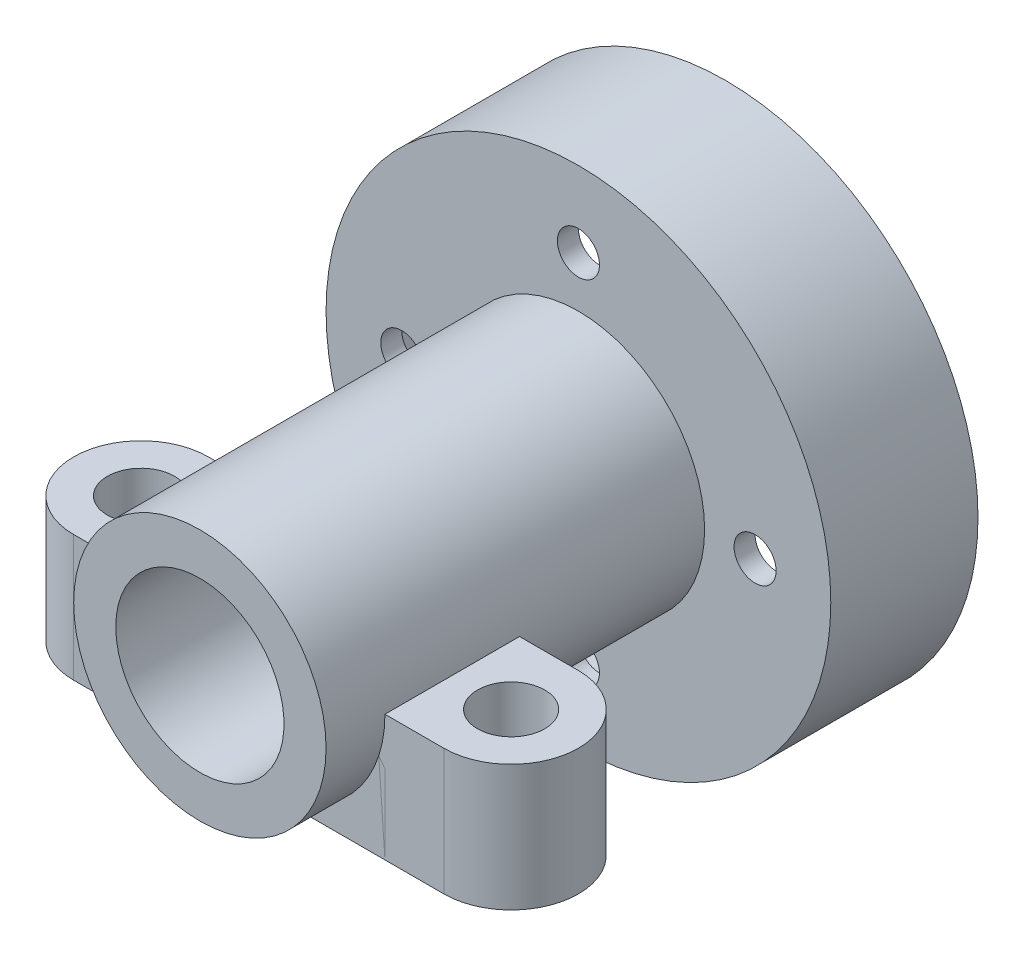
ISO-10303-21;
HEADER;
FILE_DESCRIPTION(('STEP AP214'),'2;1');
FILE_NAME('part.step','',(''),(''),'','','');
FILE_SCHEMA(('AUTOMOTIVE_DESIGN { 1 0 10303 214 1 1 1 1 }'));
ENDSEC;
DATA;
#1=APPLICATION_CONTEXT('core data for automotive mechanical design processes');
#2=APPLICATION_PROTOCOL_DEFINITION('international standard','automotive_design',2000,#1);
#3=PRODUCT_CONTEXT('',#1,'mechanical');
#4=PRODUCT('Part','Part','',(#3));
#5=PRODUCT_RELATED_PRODUCT_CATEGORY('part','',(#4));
#6=PRODUCT_DEFINITION_FORMATION('','',#4);
#7=PRODUCT_DEFINITION_CONTEXT('part definition',#1,'design');
#8=PRODUCT_DEFINITION('design','',#6,#7);
#9=PRODUCT_DEFINITION_SHAPE('','',#8);
#10=(LENGTH_UNIT() NAMED_UNIT(*) SI_UNIT(.MILLI.,.METRE.));
#11=(NAMED_UNIT(*) PLANE_ANGLE_UNIT() SI_UNIT($,.RADIAN.));
#12=(NAMED_UNIT(*) SI_UNIT($,.STERADIAN.) SOLID_ANGLE_UNIT());
#13=UNCERTAINTY_MEASURE_WITH_UNIT(LENGTH_MEASURE(1.E-05),#10,'distance_accuracy_value','');
#14=(GEOMETRIC_REPRESENTATION_CONTEXT(3) GLOBAL_UNCERTAINTY_ASSIGNED_CONTEXT((#13)) GLOBAL_UNIT_ASSIGNED_CONTEXT((#10,
#11,#12)) REPRESENTATION_CONTEXT('',''));
#15=CARTESIAN_POINT('',(0.,0.,0.));
#16=DIRECTION('',(0.,0.,1.));
#17=DIRECTION('',(1.,0.,0.));
#18=AXIS2_PLACEMENT_3D('',#15,#16,#17);
#19=CARTESIAN_POINT('',(0.,0.,81.));
#20=DIRECTION('',(0.,0.,1.));
#21=DIRECTION('',(1.,0.,0.));
#22=AXIS2_PLACEMENT_3D('',#19,#20,#21);
#23=CYLINDRICAL_SURFACE('',#22,30.);
#24=CARTESIAN_POINT('',(0.,0.,111.));
#25=DIRECTION('',(0.,0.,1.));
#26=DIRECTION('',(1.,0.,0.));
#27=AXIS2_PLACEMENT_3D('',#24,#25,#26);
#28=CIRCLE('',#27,30.);
#29=CARTESIAN_POINT('',(0.,-30.,111.));
#30=VERTEX_POINT('',#29);
#31=CARTESIAN_POINT('',(30.,0.,111.));
#32=VERTEX_POINT('',#31);
#33=EDGE_CURVE('E13',#30,#32,#28,.T.);
#34=ORIENTED_EDGE('',*,*,#33,.T.);
#35=DIRECTION('',(0.,0.,1.));
#36=VECTOR('',#35,1.);
#37=CARTESIAN_POINT('',(30.,0.,81.));
#38=LINE('',#37,#36);
#39=CARTESIAN_POINT('',(30.,0.,81.));
#40=VERTEX_POINT('',#39);
#41=EDGE_CURVE('E136',#40,#32,#38,.T.);
#42=ORIENTED_EDGE('',*,*,#41,.F.);
#43=CARTESIAN_POINT('',(0.,0.,81.));
#44=DIRECTION('',(0.,0.,1.));
#45=DIRECTION('',(1.,0.,0.));
#46=AXIS2_PLACEMENT_3D('',#43,#44,#45);
#47=CIRCLE('',#46,30.);
#48=CARTESIAN_POINT('',(0.,-30.,81.));
#49=VERTEX_POINT('',#48);
#50=EDGE_CURVE('E140',#49,#40,#47,.T.);
#51=ORIENTED_EDGE('',*,*,#50,.F.);
#52=DIRECTION('',(0.,0.,1.));
#53=VECTOR('',#52,1.);
#54=CARTESIAN_POINT('',(0.,-30.,81.));
#55=LINE('',#54,#53);
#56=EDGE_CURVE('E95',#49,#30,#55,.T.);
#57=ORIENTED_EDGE('',*,*,#56,.T.);
#58=EDGE_LOOP('',(#34,#42,#51,#57));
#59=FACE_BOUND('',#58,.T.);
#60=ADVANCED_FACE('F89',(#59),#23,.F.);
#61=CARTESIAN_POINT('',(30.,0.,81.));
#62=DIRECTION('',(-1.,0.,0.));
#63=DIRECTION('',(0.,0.,1.));
#64=AXIS2_PLACEMENT_3D('',#61,#62,#63);
#65=PLANE('',#64);
#66=DIRECTION('',(0.,-1.,0.));
#67=VECTOR('',#66,1.);
#68=CARTESIAN_POINT('',(30.,0.,111.));
#69=LINE('',#68,#67);
#70=CARTESIAN_POINT('',(30.,-30.,111.));
#71=VERTEX_POINT('',#70);
#72=EDGE_CURVE('E132',#32,#71,#69,.T.);
#73=ORIENTED_EDGE('',*,*,#72,.T.);
#74=DIRECTION('',(0.,0.,1.));
#75=VECTOR('',#74,1.);
#76=CARTESIAN_POINT('',(30.,-30.,81.));
#77=LINE('',#76,#75);
#78=CARTESIAN_POINT('',(30.,-30.,81.));
#79=VERTEX_POINT('',#78);
#80=EDGE_CURVE('E107',#79,#71,#77,.T.);
#81=ORIENTED_EDGE('',*,*,#80,.F.);
#82=DIRECTION('',(0.,-1.,0.));
#83=VECTOR('',#82,1.);
#84=CARTESIAN_POINT('',(30.,0.,81.));
#85=LINE('',#84,#83);
#86=EDGE_CURVE('E119',#40,#79,#85,.T.);
#87=ORIENTED_EDGE('',*,*,#86,.F.);
#88=ORIENTED_EDGE('',*,*,#41,.T.);
#89=EDGE_LOOP('',(#73,#81,#87,#88));
#90=FACE_BOUND('',#89,.T.);
#91=ADVANCED_FACE('F147',(#90),#65,.F.);
#92=CARTESIAN_POINT('',(0.,-30.,81.));
#93=DIRECTION('',(0.,-1.,0.));
#94=DIRECTION('',(0.,0.,-1.));
#95=AXIS2_PLACEMENT_3D('',#92,#93,#94);
#96=PLANE('',#95);
#97=DIRECTION('',(1.,0.,0.));
#98=VECTOR('',#97,1.);
#99=CARTESIAN_POINT('',(0.,-30.,111.));
#100=LINE('',#99,#98);
#101=EDGE_CURVE('E99',#30,#71,#100,.T.);
#102=ORIENTED_EDGE('',*,*,#101,.F.);
#103=ORIENTED_EDGE('',*,*,#56,.F.);
#104=DIRECTION('',(1.,0.,0.));
#105=VECTOR('',#104,1.);
#106=CARTESIAN_POINT('',(0.,-30.,81.));
#107=LINE('',#106,#105);
#108=EDGE_CURVE('E123',#49,#79,#107,.T.);
#109=ORIENTED_EDGE('',*,*,#108,.T.);
#110=ORIENTED_EDGE('',*,*,#80,.T.);
#111=EDGE_LOOP('',(#102,#103,#109,#110));
#112=FACE_BOUND('',#111,.T.);
#113=ADVANCED_FACE('F133',(#112),#96,.T.);
#114=CARTESIAN_POINT('',(0.,0.,81.));
#115=DIRECTION('',(0.,0.,1.));
#116=DIRECTION('',(1.,0.,0.));
#117=AXIS2_PLACEMENT_3D('',#114,#115,#116);
#118=PLANE('',#117);
#119=ORIENTED_EDGE('',*,*,#50,.T.);
#120=ORIENTED_EDGE('',*,*,#86,.T.);
#121=ORIENTED_EDGE('',*,*,#108,.F.);
#122=EDGE_LOOP('',(#119,#120,#121));
#123=FACE_BOUND('',#122,.T.);
#124=ADVANCED_FACE('F94',(#123),#118,.F.);
#125=CARTESIAN_POINT('',(0.,0.,111.));
#126=DIRECTION('',(0.,0.,1.));
#127=DIRECTION('',(1.,0.,0.));
#128=AXIS2_PLACEMENT_3D('',#125,#126,#127);
#129=PLANE('',#128);
#130=ORIENTED_EDGE('',*,*,#33,.F.);
#131=ORIENTED_EDGE('',*,*,#101,.T.);
#132=ORIENTED_EDGE('',*,*,#72,.F.);
#133=EDGE_LOOP('',(#130,#131,#132));
#134=FACE_BOUND('',#133,.T.);
#135=ADVANCED_FACE('F138',(#134),#129,.T.);
#136=CLOSED_SHELL('',(#60,#91,#113,#124,#135));
#137=MANIFOLD_SOLID_BREP('B2',#136);
#138=CARTESIAN_POINT('',(0.,0.,81.));
#139=DIRECTION('',(0.,0.,1.));
#140=DIRECTION('',(1.,0.,0.));
#141=AXIS2_PLACEMENT_3D('',#138,#139,#140);
#142=CYLINDRICAL_SURFACE('',#141,30.);
#143=CARTESIAN_POINT('',(0.,0.,111.));
#144=DIRECTION('',(0.,0.,1.));
#145=DIRECTION('',(1.,0.,0.));
#146=AXIS2_PLACEMENT_3D('',#143,#144,#145);
#147=CIRCLE('',#146,30.);
#148=CARTESIAN_POINT('',(-30.,0.,111.));
#149=VERTEX_POINT('',#148);
#150=CARTESIAN_POINT('',(0.,-30.,111.));
#151=VERTEX_POINT('',#150);
#152=EDGE_CURVE('E242',#149,#151,#147,.T.);
#153=ORIENTED_EDGE('',*,*,#152,.T.);
#154=DIRECTION('',(0.,0.,1.));
#155=VECTOR('',#154,1.);
#156=CARTESIAN_POINT('',(0.,-30.,81.));
#157=LINE('',#156,#155);
#158=CARTESIAN_POINT('',(0.,-30.,81.));
#159=VERTEX_POINT('',#158);
#160=EDGE_CURVE('E86',#159,#151,#157,.T.);
#161=ORIENTED_EDGE('',*,*,#160,.F.);
#162=CARTESIAN_POINT('',(0.,0.,81.));
#163=DIRECTION('',(0.,0.,1.));
#164=DIRECTION('',(1.,0.,0.));
#165=AXIS2_PLACEMENT_3D('',#162,#163,#164);
#166=CIRCLE('',#165,30.);
#167=CARTESIAN_POINT('',(-30.,0.,81.));
#168=VERTEX_POINT('',#167);
#169=EDGE_CURVE('E250',#168,#159,#166,.T.);
#170=ORIENTED_EDGE('',*,*,#169,.F.);
#171=DIRECTION('',(0.,0.,1.));
#172=VECTOR('',#171,1.);
#173=CARTESIAN_POINT('',(-30.,0.,81.));
#174=LINE('',#173,#172);
#175=EDGE_CURVE('E202',#168,#149,#174,.T.);
#176=ORIENTED_EDGE('',*,*,#175,.T.);
#177=EDGE_LOOP('',(#153,#161,#170,#176));
#178=FACE_BOUND('',#177,.T.);
#179=ADVANCED_FACE('F199',(#178),#142,.F.);
#180=CARTESIAN_POINT('',(0.,-30.,81.));
#181=DIRECTION('',(0.,-1.,0.));
#182=DIRECTION('',(0.,0.,-1.));
#183=AXIS2_PLACEMENT_3D('',#180,#181,#182);
#184=PLANE('',#183);
#185=DIRECTION('',(1.,0.,0.));
#186=VECTOR('',#185,1.);
#187=CARTESIAN_POINT('',(0.,-30.,111.));
#188=LINE('',#187,#186);
#189=CARTESIAN_POINT('',(-30.,-30.,111.));
#190=VERTEX_POINT('',#189);
#191=EDGE_CURVE('E243',#190,#151,#188,.T.);
#192=ORIENTED_EDGE('',*,*,#191,.F.);
#193=DIRECTION('',(0.,0.,1.));
#194=VECTOR('',#193,1.);
#195=CARTESIAN_POINT('',(-30.,-30.,81.));
#196=LINE('',#195,#194);
#197=CARTESIAN_POINT('',(-30.,-30.,81.));
#198=VERTEX_POINT('',#197);
#199=EDGE_CURVE('E209',#198,#190,#196,.T.);
#200=ORIENTED_EDGE('',*,*,#199,.F.);
#201=DIRECTION('',(1.,0.,0.));
#202=VECTOR('',#201,1.);
#203=CARTESIAN_POINT('',(0.,-30.,81.));
#204=LINE('',#203,#202);
#205=EDGE_CURVE('E254',#198,#159,#204,.T.);
#206=ORIENTED_EDGE('',*,*,#205,.T.);
#207=ORIENTED_EDGE('',*,*,#160,.T.);
#208=EDGE_LOOP('',(#192,#200,#206,#207));
#209=FACE_BOUND('',#208,.T.);
#210=ADVANCED_FACE('F246',(#209),#184,.T.);
#211=CARTESIAN_POINT('',(-30.,0.,81.));
#212=DIRECTION('',(-1.,0.,0.));
#213=DIRECTION('',(0.,0.,1.));
#214=AXIS2_PLACEMENT_3D('',#211,#212,#213);
#215=PLANE('',#214);
#216=DIRECTION('',(0.,-1.,0.));
#217=VECTOR('',#216,1.);
#218=CARTESIAN_POINT('',(-30.,0.,111.));
#219=LINE('',#218,#217);
#220=EDGE_CURVE('E234',#149,#190,#219,.T.);
#221=ORIENTED_EDGE('',*,*,#220,.F.);
#222=ORIENTED_EDGE('',*,*,#175,.F.);
#223=DIRECTION('',(0.,-1.,0.));
#224=VECTOR('',#223,1.);
#225=CARTESIAN_POINT('',(-30.,0.,81.));
#226=LINE('',#225,#224);
#227=EDGE_CURVE('E236',#168,#198,#226,.T.);
#228=ORIENTED_EDGE('',*,*,#227,.T.);
#229=ORIENTED_EDGE('',*,*,#199,.T.);
#230=EDGE_LOOP('',(#221,#222,#228,#229));
#231=FACE_BOUND('',#230,.T.);
#232=ADVANCED_FACE('F231',(#231),#215,.T.);
#233=CARTESIAN_POINT('',(0.,0.,81.));
#234=DIRECTION('',(0.,0.,1.));
#235=DIRECTION('',(1.,0.,0.));
#236=AXIS2_PLACEMENT_3D('',#233,#234,#235);
#237=PLANE('',#236);
#238=ORIENTED_EDGE('',*,*,#169,.T.);
#239=ORIENTED_EDGE('',*,*,#205,.F.);
#240=ORIENTED_EDGE('',*,*,#227,.F.);
#241=EDGE_LOOP('',(#238,#239,#240));
#242=FACE_BOUND('',#241,.T.);
#243=ADVANCED_FACE('F257',(#242),#237,.F.);
#244=CARTESIAN_POINT('',(0.,0.,111.));
#245=DIRECTION('',(0.,0.,1.));
#246=DIRECTION('',(1.,0.,0.));
#247=AXIS2_PLACEMENT_3D('',#244,#245,#246);
#248=PLANE('',#247);
#249=ORIENTED_EDGE('',*,*,#152,.F.);
#250=ORIENTED_EDGE('',*,*,#220,.T.);
#251=ORIENTED_EDGE('',*,*,#191,.T.);
#252=EDGE_LOOP('',(#249,#250,#251));
#253=FACE_BOUND('',#252,.T.);
#254=ADVANCED_FACE('F245',(#253),#248,.T.);
#255=CLOSED_SHELL('',(#179,#210,#232,#243,#254));
#256=MANIFOLD_SOLID_BREP('B7',#255);
#257=CARTESIAN_POINT('',(0.,0.,65.));
#258=DIRECTION('',(0.,0.,-1.));
#259=DIRECTION('',(-1.,0.,0.));
#260=AXIS2_PLACEMENT_3D('',#257,#258,#259);
#261=CYLINDRICAL_SURFACE('',#260,30.);
#262=CARTESIAN_POINT('',(0.,0.,35.));
#263=DIRECTION('',(0.,0.,1.));
#264=DIRECTION('',(1.,0.,0.));
#265=AXIS2_PLACEMENT_3D('',#262,#263,#264);
#266=CIRCLE('',#265,30.);
#267=CARTESIAN_POINT('',(30.,0.,35.));
#268=VERTEX_POINT('',#267);
#269=EDGE_CURVE('E362',#268,#268,#266,.T.);
#270=ORIENTED_EDGE('',*,*,#269,.T.);
#271=EDGE_LOOP('',(#270));
#272=FACE_BOUND('',#271,.T.);
#273=CARTESIAN_POINT('',(0.,0.,125.));
#274=DIRECTION('',(0.,0.,1.));
#275=DIRECTION('',(1.,0.,0.));
#276=AXIS2_PLACEMENT_3D('',#273,#274,#275);
#277=CIRCLE('',#276,30.);
#278=CARTESIAN_POINT('',(30.,0.,125.));
#279=VERTEX_POINT('',#278);
#280=EDGE_CURVE('E401',#279,#279,#277,.T.);
#281=ORIENTED_EDGE('',*,*,#280,.F.);
#282=EDGE_LOOP('',(#281));
#283=FACE_BOUND('',#282,.T.);
#284=CARTESIAN_POINT('',(0.,0.,79.));
#285=DIRECTION('',(0.,0.,1.));
#286=DIRECTION('',(1.,0.,0.));
#287=AXIS2_PLACEMENT_3D('',#284,#285,#286);
#288=CIRCLE('',#287,30.);
#289=CARTESIAN_POINT('',(-30.,0.,79.));
#290=VERTEX_POINT('',#289);
#291=CARTESIAN_POINT('',(0.,-30.,79.));
#292=VERTEX_POINT('',#291);
#293=EDGE_CURVE('E432',#290,#292,#288,.T.);
#294=ORIENTED_EDGE('',*,*,#293,.F.);
#295=DIRECTION('',(0.,0.,1.));
#296=VECTOR('',#295,1.);
#297=CARTESIAN_POINT('',(-30.,0.,79.));
#298=LINE('',#297,#296);
#299=CARTESIAN_POINT('',(-30.,0.,111.));
#300=VERTEX_POINT('',#299);
#301=EDGE_CURVE('E430',#290,#300,#298,.T.);
#302=ORIENTED_EDGE('',*,*,#301,.T.);
#303=CARTESIAN_POINT('',(0.,0.,111.));
#304=DIRECTION('',(0.,0.,1.));
#305=DIRECTION('',(1.,0.,0.));
#306=AXIS2_PLACEMENT_3D('',#303,#304,#305);
#307=CIRCLE('',#306,30.);
#308=CARTESIAN_POINT('',(0.,-30.,111.));
#309=VERTEX_POINT('',#308);
#310=EDGE_CURVE('E434',#300,#309,#307,.T.);
#311=ORIENTED_EDGE('',*,*,#310,.T.);
#312=CARTESIAN_POINT('',(0.,0.,111.));
#313=DIRECTION('',(0.,0.,1.));
#314=DIRECTION('',(1.,0.,0.));
#315=AXIS2_PLACEMENT_3D('',#312,#313,#314);
#316=CIRCLE('',#315,30.);
#317=CARTESIAN_POINT('',(30.,0.,111.));
#318=VERTEX_POINT('',#317);
#319=EDGE_CURVE('E326',#309,#318,#316,.T.);
#320=ORIENTED_EDGE('',*,*,#319,.T.);
#321=DIRECTION('',(0.,0.,1.));
#322=VECTOR('',#321,1.);
#323=CARTESIAN_POINT('',(30.,0.,79.));
#324=LINE('',#323,#322);
#325=CARTESIAN_POINT('',(30.,0.,79.));
#326=VERTEX_POINT('',#325);
#327=EDGE_CURVE('E350',#326,#318,#324,.T.);
#328=ORIENTED_EDGE('',*,*,#327,.F.);
#329=CARTESIAN_POINT('',(0.,0.,79.));
#330=DIRECTION('',(0.,0.,1.));
#331=DIRECTION('',(1.,0.,0.));
#332=AXIS2_PLACEMENT_3D('',#329,#330,#331);
#333=CIRCLE('',#332,30.);
#334=EDGE_CURVE('E363',#292,#326,#333,.T.);
#335=ORIENTED_EDGE('',*,*,#334,.F.);
#336=EDGE_LOOP('',(#294,#302,#311,#320,#328,#335));
#337=FACE_BOUND('',#336,.T.);
#338=ADVANCED_FACE('F296',(#272,#283,#337),#261,.T.);
#339=CARTESIAN_POINT('',(44.,-30.,95.));
#340=DIRECTION('',(0.,1.,0.));
#341=DIRECTION('',(0.,0.,1.));
#342=AXIS2_PLACEMENT_3D('',#339,#340,#341);
#343=CYLINDRICAL_SURFACE('',#342,16.);
#344=CARTESIAN_POINT('',(44.,0.,95.));
#345=DIRECTION('',(0.,1.,0.));
#346=DIRECTION('',(0.,0.,1.));
#347=AXIS2_PLACEMENT_3D('',#344,#345,#346);
#348=CIRCLE('',#347,16.);
#349=CARTESIAN_POINT('',(44.,0.,111.));
#350=VERTEX_POINT('',#349);
#351=CARTESIAN_POINT('',(44.,0.,79.));
#352=VERTEX_POINT('',#351);
#353=EDGE_CURVE('E339',#350,#352,#348,.T.);
#354=ORIENTED_EDGE('',*,*,#353,.F.);
#355=DIRECTION('',(0.,1.,0.));
#356=VECTOR('',#355,1.);
#357=CARTESIAN_POINT('',(44.,-30.,111.));
#358=LINE('',#357,#356);
#359=CARTESIAN_POINT('',(44.,-30.,111.));
#360=VERTEX_POINT('',#359);
#361=EDGE_CURVE('E196',#360,#350,#358,.T.);
#362=ORIENTED_EDGE('',*,*,#361,.F.);
#363=CARTESIAN_POINT('',(44.,-30.,95.));
#364=DIRECTION('',(0.,1.,0.));
#365=DIRECTION('',(0.,0.,1.));
#366=AXIS2_PLACEMENT_3D('',#363,#364,#365);
#367=CIRCLE('',#366,16.);
#368=CARTESIAN_POINT('',(44.,-30.,79.));
#369=VERTEX_POINT('',#368);
#370=EDGE_CURVE('E346',#360,#369,#367,.T.);
#371=ORIENTED_EDGE('',*,*,#370,.T.);
#372=DIRECTION('',(0.,1.,0.));
#373=VECTOR('',#372,1.);
#374=CARTESIAN_POINT('',(44.,-30.,79.));
#375=LINE('',#374,#373);
#376=EDGE_CURVE('E305',#369,#352,#375,.T.);
#377=ORIENTED_EDGE('',*,*,#376,.T.);
#378=EDGE_LOOP('',(#354,#362,#371,#377));
#379=FACE_BOUND('',#378,.T.);
#380=ADVANCED_FACE('F297',(#379),#343,.T.);
#381=CARTESIAN_POINT('',(30.,-30.,111.));
#382=DIRECTION('',(0.,0.,1.));
#383=DIRECTION('',(1.,0.,0.));
#384=AXIS2_PLACEMENT_3D('',#381,#382,#383);
#385=PLANE('',#384);
#386=DIRECTION('',(1.,0.,0.));
#387=VECTOR('',#386,1.);
#388=CARTESIAN_POINT('',(30.,0.,111.));
#389=LINE('',#388,#387);
#390=EDGE_CURVE('E331',#318,#350,#389,.T.);
#391=ORIENTED_EDGE('',*,*,#390,.F.);
#392=ORIENTED_EDGE('',*,*,#319,.F.);
#393=DIRECTION('',(1.,0.,0.));
#394=VECTOR('',#393,1.);
#395=CARTESIAN_POINT('',(30.,-30.,111.));
#396=LINE('',#395,#394);
#397=EDGE_CURVE('E340',#309,#360,#396,.T.);
#398=ORIENTED_EDGE('',*,*,#397,.T.);
#399=ORIENTED_EDGE('',*,*,#361,.T.);
#400=EDGE_LOOP('',(#391,#392,#398,#399));
#401=FACE_BOUND('',#400,.T.);
#402=ADVANCED_FACE('F332',(#401),#385,.T.);
#403=CARTESIAN_POINT('',(44.,-30.,79.));
#404=DIRECTION('',(0.,0.,-1.));
#405=DIRECTION('',(-1.,0.,0.));
#406=AXIS2_PLACEMENT_3D('',#403,#404,#405);
#407=PLANE('',#406);
#408=DIRECTION('',(-1.,0.,0.));
#409=VECTOR('',#408,1.);
#410=CARTESIAN_POINT('',(44.,0.,79.));
#411=LINE('',#410,#409);
#412=EDGE_CURVE('E344',#352,#326,#411,.T.);
#413=ORIENTED_EDGE('',*,*,#412,.F.);
#414=ORIENTED_EDGE('',*,*,#376,.F.);
#415=DIRECTION('',(-1.,0.,0.));
#416=VECTOR('',#415,1.);
#417=CARTESIAN_POINT('',(44.,-30.,79.));
#418=LINE('',#417,#416);
#419=EDGE_CURVE('E349',#369,#292,#418,.T.);
#420=ORIENTED_EDGE('',*,*,#419,.T.);
#421=ORIENTED_EDGE('',*,*,#334,.T.);
#422=EDGE_LOOP('',(#413,#414,#420,#421));
#423=FACE_BOUND('',#422,.T.);
#424=ADVANCED_FACE('F508',(#423),#407,.T.);
#425=CARTESIAN_POINT('',(44.,-30.,95.));
#426=DIRECTION('',(0.,1.,0.));
#427=DIRECTION('',(0.,0.,1.));
#428=AXIS2_PLACEMENT_3D('',#425,#426,#427);
#429=PLANE('',#428);
#430=CARTESIAN_POINT('',(44.,-30.,95.));
#431=DIRECTION('',(0.,1.,0.));
#432=DIRECTION('',(0.,0.,1.));
#433=AXIS2_PLACEMENT_3D('',#430,#431,#432);
#434=CIRCLE('',#433,8.);
#435=CARTESIAN_POINT('',(44.,-30.,103.));
#436=VERTEX_POINT('',#435);
#437=EDGE_CURVE('E341',#436,#436,#434,.T.);
#438=ORIENTED_EDGE('',*,*,#437,.T.);
#439=EDGE_LOOP('',(#438));
#440=FACE_BOUND('',#439,.T.);
#441=ORIENTED_EDGE('',*,*,#370,.F.);
#442=ORIENTED_EDGE('',*,*,#397,.F.);
#443=DIRECTION('',(-1.,0.,0.));
#444=VECTOR('',#443,1.);
#445=CARTESIAN_POINT('',(0.,-30.,111.));
#446=LINE('',#445,#444);
#447=CARTESIAN_POINT('',(-44.,-30.,111.));
#448=VERTEX_POINT('',#447);
#449=EDGE_CURVE('E431',#309,#448,#446,.T.);
#450=ORIENTED_EDGE('',*,*,#449,.T.);
#451=CARTESIAN_POINT('',(-44.,-30.,95.));
#452=DIRECTION('',(0.,1.,0.));
#453=DIRECTION('',(0.,0.,-1.));
#454=AXIS2_PLACEMENT_3D('',#451,#452,#453);
#455=CIRCLE('',#454,16.);
#456=CARTESIAN_POINT('',(-44.,-30.,79.));
#457=VERTEX_POINT('',#456);
#458=EDGE_CURVE('E444',#457,#448,#455,.T.);
#459=ORIENTED_EDGE('',*,*,#458,.F.);
#460=DIRECTION('',(-1.,0.,0.));
#461=VECTOR('',#460,1.);
#462=CARTESIAN_POINT('',(0.,-30.,79.));
#463=LINE('',#462,#461);
#464=EDGE_CURVE('E427',#292,#457,#463,.T.);
#465=ORIENTED_EDGE('',*,*,#464,.F.);
#466=ORIENTED_EDGE('',*,*,#419,.F.);
#467=EDGE_LOOP('',(#441,#442,#450,#459,#465,#466));
#468=FACE_BOUND('',#467,.T.);
#469=CARTESIAN_POINT('',(-44.,-30.,95.));
#470=DIRECTION('',(0.,1.,0.));
#471=DIRECTION('',(0.,0.,-1.));
#472=AXIS2_PLACEMENT_3D('',#469,#470,#471);
#473=CIRCLE('',#472,8.);
#474=CARTESIAN_POINT('',(-44.,-30.,87.));
#475=VERTEX_POINT('',#474);
#476=EDGE_CURVE('E460',#475,#475,#473,.T.);
#477=ORIENTED_EDGE('',*,*,#476,.T.);
#478=EDGE_LOOP('',(#477));
#479=FACE_BOUND('',#478,.T.);
#480=ADVANCED_FACE('F467',(#440,#468,#479),#429,.F.);
#481=CARTESIAN_POINT('',(44.,0.,95.));
#482=DIRECTION('',(0.,1.,0.));
#483=DIRECTION('',(0.,0.,1.));
#484=AXIS2_PLACEMENT_3D('',#481,#482,#483);
#485=PLANE('',#484);
#486=CARTESIAN_POINT('',(44.,0.,95.));
#487=DIRECTION('',(0.,1.,0.));
#488=DIRECTION('',(0.,0.,1.));
#489=AXIS2_PLACEMENT_3D('',#486,#487,#488);
#490=CIRCLE('',#489,8.);
#491=CARTESIAN_POINT('',(44.,0.,103.));
#492=VERTEX_POINT('',#491);
#493=EDGE_CURVE('E356',#492,#492,#490,.T.);
#494=ORIENTED_EDGE('',*,*,#493,.F.);
#495=EDGE_LOOP('',(#494));
#496=FACE_BOUND('',#495,.T.);
#497=ORIENTED_EDGE('',*,*,#353,.T.);
#498=ORIENTED_EDGE('',*,*,#412,.T.);
#499=ORIENTED_EDGE('',*,*,#327,.T.);
#500=ORIENTED_EDGE('',*,*,#390,.T.);
#501=EDGE_LOOP('',(#497,#498,#499,#500));
#502=FACE_BOUND('',#501,.T.);
#503=ADVANCED_FACE('F348',(#496,#502),#485,.T.);
#504=CARTESIAN_POINT('',(44.,-30.,95.));
#505=DIRECTION('',(0.,1.,0.));
#506=DIRECTION('',(0.,0.,1.));
#507=AXIS2_PLACEMENT_3D('',#504,#505,#506);
#508=CYLINDRICAL_SURFACE('',#507,8.);
#509=ORIENTED_EDGE('',*,*,#437,.F.);
#510=EDGE_LOOP('',(#509));
#511=FACE_BOUND('',#510,.T.);
#512=ORIENTED_EDGE('',*,*,#493,.T.);
#513=EDGE_LOOP('',(#512));
#514=FACE_BOUND('',#513,.T.);
#515=ADVANCED_FACE('F582',(#511,#514),#508,.F.);
#516=CARTESIAN_POINT('',(0.,0.,65.));
#517=DIRECTION('',(0.,0.,1.));
#518=DIRECTION('',(1.,0.,0.));
#519=AXIS2_PLACEMENT_3D('',#516,#517,#518);
#520=PLANE('',#519);
#521=CARTESIAN_POINT('',(0.,0.,65.));
#522=DIRECTION('',(0.,0.,1.));
#523=DIRECTION('',(1.,0.,0.));
#524=AXIS2_PLACEMENT_3D('',#521,#522,#523);
#525=CIRCLE('',#524,12.5);
#526=CARTESIAN_POINT('',(12.5,0.,65.));
#527=VERTEX_POINT('',#526);
#528=EDGE_CURVE('E425',#527,#527,#525,.T.);
#529=ORIENTED_EDGE('',*,*,#528,.F.);
#530=EDGE_LOOP('',(#529));
#531=FACE_BOUND('',#530,.T.);
#532=CARTESIAN_POINT('',(0.,0.,65.));
#533=DIRECTION('',(0.,0.,-1.));
#534=DIRECTION('',(1.,0.,0.));
#535=AXIS2_PLACEMENT_3D('',#532,#533,#534);
#536=CIRCLE('',#535,20.);
#537=CARTESIAN_POINT('',(-20.,0.,65.));
#538=VERTEX_POINT('',#537);
#539=EDGE_CURVE('E411',#538,#538,#536,.T.);
#540=ORIENTED_EDGE('',*,*,#539,.F.);
#541=EDGE_LOOP('',(#540));
#542=FACE_BOUND('',#541,.T.);
#543=ADVANCED_FACE('F534',(#531,#542),#520,.T.);
#544=CARTESIAN_POINT('',(0.,0.,35.));
#545=DIRECTION('',(0.,0.,-1.));
#546=DIRECTION('',(-1.,0.,0.));
#547=AXIS2_PLACEMENT_3D('',#544,#545,#546);
#548=CYLINDRICAL_SURFACE('',#547,60.);
#549=CARTESIAN_POINT('',(0.,0.,35.));
#550=DIRECTION('',(0.,0.,1.));
#551=DIRECTION('',(1.,0.,0.));
#552=AXIS2_PLACEMENT_3D('',#549,#550,#551);
#553=CIRCLE('',#552,60.);
#554=CARTESIAN_POINT('',(60.,0.,35.));
#555=VERTEX_POINT('',#554);
#556=EDGE_CURVE('E383',#555,#555,#553,.T.);
#557=ORIENTED_EDGE('',*,*,#556,.F.);
#558=EDGE_LOOP('',(#557));
#559=FACE_BOUND('',#558,.T.);
#560=CARTESIAN_POINT('',(0.,0.,0.));
#561=DIRECTION('',(0.,0.,1.));
#562=DIRECTION('',(1.,0.,0.));
#563=AXIS2_PLACEMENT_3D('',#560,#561,#562);
#564=CIRCLE('',#563,60.);
#565=CARTESIAN_POINT('',(60.,0.,0.));
#566=VERTEX_POINT('',#565);
#567=EDGE_CURVE('E385',#566,#566,#564,.T.);
#568=ORIENTED_EDGE('',*,*,#567,.T.);
#569=EDGE_LOOP('',(#568));
#570=FACE_BOUND('',#569,.T.);
#571=ADVANCED_FACE('F572',(#559,#570),#548,.T.);
#572=CARTESIAN_POINT('',(0.,0.,35.));
#573=DIRECTION('',(0.,0.,1.));
#574=DIRECTION('',(1.,0.,0.));
#575=AXIS2_PLACEMENT_3D('',#572,#573,#574);
#576=PLANE('',#575);
#577=ORIENTED_EDGE('',*,*,#269,.F.);
#578=EDGE_LOOP('',(#577));
#579=FACE_BOUND('',#578,.T.);
#580=CARTESIAN_POINT('',(42.,0.,35.));
#581=DIRECTION('',(0.,0.,1.));
#582=DIRECTION('',(1.,0.,0.));
#583=AXIS2_PLACEMENT_3D('',#580,#581,#582);
#584=CIRCLE('',#583,5.);
#585=CARTESIAN_POINT('',(47.,0.,35.));
#586=VERTEX_POINT('',#585);
#587=EDGE_CURVE('E382',#586,#586,#584,.T.);
#588=ORIENTED_EDGE('',*,*,#587,.F.);
#589=EDGE_LOOP('',(#588));
#590=FACE_BOUND('',#589,.T.);
#591=CARTESIAN_POINT('',(0.,-42.,35.));
#592=DIRECTION('',(0.,0.,1.));
#593=DIRECTION('',(1.,0.,0.));
#594=AXIS2_PLACEMENT_3D('',#591,#592,#593);
#595=CIRCLE('',#594,4.99999999999995);
#596=CARTESIAN_POINT('',(4.99999999999997,-42.,35.));
#597=VERTEX_POINT('',#596);
#598=EDGE_CURVE('E407',#597,#597,#595,.T.);
#599=ORIENTED_EDGE('',*,*,#598,.F.);
#600=EDGE_LOOP('',(#599));
#601=FACE_BOUND('',#600,.T.);
#602=CARTESIAN_POINT('',(-42.,2.93284432462823E-13,35.));
#603=DIRECTION('',(0.,0.,1.));
#604=DIRECTION('',(1.,0.,0.));
#605=AXIS2_PLACEMENT_3D('',#602,#603,#604);
#606=CIRCLE('',#605,4.99999999999999);
#607=CARTESIAN_POINT('',(-37.,2.93284432462823E-13,35.));
#608=VERTEX_POINT('',#607);
#609=EDGE_CURVE('E405',#608,#608,#606,.T.);
#610=ORIENTED_EDGE('',*,*,#609,.F.);
#611=EDGE_LOOP('',(#610));
#612=FACE_BOUND('',#611,.T.);
#613=CARTESIAN_POINT('',(0.,42.,35.));
#614=DIRECTION('',(0.,0.,1.));
#615=DIRECTION('',(1.,0.,0.));
#616=AXIS2_PLACEMENT_3D('',#613,#614,#615);
#617=CIRCLE('',#616,4.99999999999987);
#618=CARTESIAN_POINT('',(4.99999999999987,42.,35.));
#619=VERTEX_POINT('',#618);
#620=EDGE_CURVE('E400',#619,#619,#617,.T.);
#621=ORIENTED_EDGE('',*,*,#620,.F.);
#622=EDGE_LOOP('',(#621));
#623=FACE_BOUND('',#622,.T.);
#624=ORIENTED_EDGE('',*,*,#556,.T.);
#625=EDGE_LOOP('',(#624));
#626=FACE_BOUND('',#625,.T.);
#627=ADVANCED_FACE('F569',(#579,#590,#601,#612,#623,#626),#576,.T.);
#628=CARTESIAN_POINT('',(0.,0.,0.));
#629=DIRECTION('',(0.,0.,1.));
#630=DIRECTION('',(1.,0.,0.));
#631=AXIS2_PLACEMENT_3D('',#628,#629,#630);
#632=PLANE('',#631);
#633=CARTESIAN_POINT('',(0.,0.,0.));
#634=DIRECTION('',(0.,0.,-1.));
#635=DIRECTION('',(-1.,0.,0.));
#636=AXIS2_PLACEMENT_3D('',#633,#634,#635);
#637=CIRCLE('',#636,55.);
#638=CARTESIAN_POINT('',(-55.,0.,0.));
#639=VERTEX_POINT('',#638);
#640=EDGE_CURVE('E386',#639,#639,#637,.T.);
#641=ORIENTED_EDGE('',*,*,#640,.F.);
#642=EDGE_LOOP('',(#641));
#643=FACE_BOUND('',#642,.T.);
#644=ORIENTED_EDGE('',*,*,#567,.F.);
#645=EDGE_LOOP('',(#644));
#646=FACE_BOUND('',#645,.T.);
#647=ADVANCED_FACE('F568',(#643,#646),#632,.F.);
#648=CARTESIAN_POINT('',(0.,0.,15.));
#649=DIRECTION('',(0.,0.,-1.));
#650=DIRECTION('',(-1.,0.,0.));
#651=AXIS2_PLACEMENT_3D('',#648,#649,#650);
#652=CYLINDRICAL_SURFACE('',#651,55.);
#653=CARTESIAN_POINT('',(0.,0.,15.));
#654=DIRECTION('',(0.,0.,-1.));
#655=DIRECTION('',(-1.,0.,0.));
#656=AXIS2_PLACEMENT_3D('',#653,#654,#655);
#657=CIRCLE('',#656,55.);
#658=CARTESIAN_POINT('',(-55.,0.,15.));
#659=VERTEX_POINT('',#658);
#660=EDGE_CURVE('E387',#659,#659,#657,.T.);
#661=ORIENTED_EDGE('',*,*,#660,.F.);
#662=EDGE_LOOP('',(#661));
#663=FACE_BOUND('',#662,.T.);
#664=ORIENTED_EDGE('',*,*,#640,.T.);
#665=EDGE_LOOP('',(#664));
#666=FACE_BOUND('',#665,.T.);
#667=ADVANCED_FACE('F562',(#663,#666),#652,.F.);
#668=CARTESIAN_POINT('',(0.,0.,15.));
#669=DIRECTION('',(0.,0.,-1.));
#670=DIRECTION('',(-1.,0.,0.));
#671=AXIS2_PLACEMENT_3D('',#668,#669,#670);
#672=PLANE('',#671);
#673=CARTESIAN_POINT('',(0.,0.,15.));
#674=DIRECTION('',(0.,0.,-1.));
#675=DIRECTION('',(-1.,0.,0.));
#676=AXIS2_PLACEMENT_3D('',#673,#674,#675);
#677=CIRCLE('',#676,50.);
#678=CARTESIAN_POINT('',(-50.,0.,15.));
#679=VERTEX_POINT('',#678);
#680=EDGE_CURVE('E371',#679,#679,#677,.T.);
#681=ORIENTED_EDGE('',*,*,#680,.F.);
#682=EDGE_LOOP('',(#681));
#683=FACE_BOUND('',#682,.T.);
#684=ORIENTED_EDGE('',*,*,#660,.T.);
#685=EDGE_LOOP('',(#684));
#686=FACE_BOUND('',#685,.T.);
#687=ADVANCED_FACE('F557',(#683,#686),#672,.T.);
#688=CARTESIAN_POINT('',(0.,0.,30.));
#689=DIRECTION('',(0.,0.,-1.));
#690=DIRECTION('',(-1.,0.,0.));
#691=AXIS2_PLACEMENT_3D('',#688,#689,#690);
#692=CYLINDRICAL_SURFACE('',#691,50.);
#693=CARTESIAN_POINT('',(0.,0.,30.));
#694=DIRECTION('',(0.,0.,-1.));
#695=DIRECTION('',(-1.,0.,0.));
#696=AXIS2_PLACEMENT_3D('',#693,#694,#695);
#697=CIRCLE('',#696,50.);
#698=CARTESIAN_POINT('',(-50.,0.,30.));
#699=VERTEX_POINT('',#698);
#700=EDGE_CURVE('E395',#699,#699,#697,.T.);
#701=ORIENTED_EDGE('',*,*,#700,.F.);
#702=EDGE_LOOP('',(#701));
#703=FACE_BOUND('',#702,.T.);
#704=ORIENTED_EDGE('',*,*,#680,.T.);
#705=EDGE_LOOP('',(#704));
#706=FACE_BOUND('',#705,.T.);
#707=ADVANCED_FACE('F558',(#703,#706),#692,.F.);
#708=CARTESIAN_POINT('',(0.,0.,30.));
#709=DIRECTION('',(0.,0.,-1.));
#710=DIRECTION('',(-1.,0.,0.));
#711=AXIS2_PLACEMENT_3D('',#708,#709,#710);
#712=PLANE('',#711);
#713=CARTESIAN_POINT('',(0.,0.,30.));
#714=DIRECTION('',(0.,0.,-1.));
#715=DIRECTION('',(-1.,0.,0.));
#716=AXIS2_PLACEMENT_3D('',#713,#714,#715);
#717=CIRCLE('',#716,12.5);
#718=CARTESIAN_POINT('',(-12.5,0.,30.));
#719=VERTEX_POINT('',#718);
#720=EDGE_CURVE('E419',#719,#719,#717,.T.);
#721=ORIENTED_EDGE('',*,*,#720,.F.);
#722=EDGE_LOOP('',(#721));
#723=FACE_BOUND('',#722,.T.);
#724=CARTESIAN_POINT('',(42.,0.,30.));
#725=DIRECTION('',(0.,0.,-1.));
#726=DIRECTION('',(-1.,0.,0.));
#727=AXIS2_PLACEMENT_3D('',#724,#725,#726);
#728=CIRCLE('',#727,5.);
#729=CARTESIAN_POINT('',(37.,0.,30.));
#730=VERTEX_POINT('',#729);
#731=EDGE_CURVE('E368',#730,#730,#728,.T.);
#732=ORIENTED_EDGE('',*,*,#731,.F.);
#733=EDGE_LOOP('',(#732));
#734=FACE_BOUND('',#733,.T.);
#735=CARTESIAN_POINT('',(0.,-42.,30.));
#736=DIRECTION('',(0.,0.,-1.));
#737=DIRECTION('',(-1.,0.,0.));
#738=AXIS2_PLACEMENT_3D('',#735,#736,#737);
#739=CIRCLE('',#738,4.99999999999995);
#740=CARTESIAN_POINT('',(-4.99999999999993,-42.,30.));
#741=VERTEX_POINT('',#740);
#742=EDGE_CURVE('E375',#741,#741,#739,.T.);
#743=ORIENTED_EDGE('',*,*,#742,.F.);
#744=EDGE_LOOP('',(#743));
#745=FACE_BOUND('',#744,.T.);
#746=CARTESIAN_POINT('',(-42.,2.93284432462823E-13,30.));
#747=DIRECTION('',(0.,0.,-1.));
#748=DIRECTION('',(-1.,0.,0.));
#749=AXIS2_PLACEMENT_3D('',#746,#747,#748);
#750=CIRCLE('',#749,4.99999999999999);
#751=CARTESIAN_POINT('',(-47.,2.93284432462823E-13,30.));
#752=VERTEX_POINT('',#751);
#753=EDGE_CURVE('E374',#752,#752,#750,.T.);
#754=ORIENTED_EDGE('',*,*,#753,.F.);
#755=EDGE_LOOP('',(#754));
#756=FACE_BOUND('',#755,.T.);
#757=CARTESIAN_POINT('',(0.,42.,30.));
#758=DIRECTION('',(0.,0.,-1.));
#759=DIRECTION('',(-1.,0.,0.));
#760=AXIS2_PLACEMENT_3D('',#757,#758,#759);
#761=CIRCLE('',#760,4.99999999999987);
#762=CARTESIAN_POINT('',(-4.99999999999988,42.,30.));
#763=VERTEX_POINT('',#762);
#764=EDGE_CURVE('E377',#763,#763,#761,.T.);
#765=ORIENTED_EDGE('',*,*,#764,.F.);
#766=EDGE_LOOP('',(#765));
#767=FACE_BOUND('',#766,.T.);
#768=ORIENTED_EDGE('',*,*,#700,.T.);
#769=EDGE_LOOP('',(#768));
#770=FACE_BOUND('',#769,.T.);
#771=ADVANCED_FACE('F552',(#723,#734,#745,#756,#767,#770),#712,.T.);
#772=CARTESIAN_POINT('',(0.,42.,20.));
#773=DIRECTION('',(0.,0.,1.));
#774=DIRECTION('',(1.,0.,0.));
#775=AXIS2_PLACEMENT_3D('',#772,#773,#774);
#776=CYLINDRICAL_SURFACE('',#775,4.99999999999987);
#777=ORIENTED_EDGE('',*,*,#764,.T.);
#778=EDGE_LOOP('',(#777));
#779=FACE_BOUND('',#778,.T.);
#780=ORIENTED_EDGE('',*,*,#620,.T.);
#781=EDGE_LOOP('',(#780));
#782=FACE_BOUND('',#781,.T.);
#783=ADVANCED_FACE('F547',(#779,#782),#776,.F.);
#784=CARTESIAN_POINT('',(-42.,2.93284432462823E-13,20.));
#785=DIRECTION('',(0.,0.,1.));
#786=DIRECTION('',(1.,0.,0.));
#787=AXIS2_PLACEMENT_3D('',#784,#785,#786);
#788=CYLINDRICAL_SURFACE('',#787,4.99999999999999);
#789=ORIENTED_EDGE('',*,*,#753,.T.);
#790=EDGE_LOOP('',(#789));
#791=FACE_BOUND('',#790,.T.);
#792=ORIENTED_EDGE('',*,*,#609,.T.);
#793=EDGE_LOOP('',(#792));
#794=FACE_BOUND('',#793,.T.);
#795=ADVANCED_FACE('F542',(#791,#794),#788,.F.);
#796=CARTESIAN_POINT('',(0.,-42.,20.));
#797=DIRECTION('',(0.,0.,1.));
#798=DIRECTION('',(1.,0.,0.));
#799=AXIS2_PLACEMENT_3D('',#796,#797,#798);
#800=CYLINDRICAL_SURFACE('',#799,4.99999999999995);
#801=ORIENTED_EDGE('',*,*,#742,.T.);
#802=EDGE_LOOP('',(#801));
#803=FACE_BOUND('',#802,.T.);
#804=ORIENTED_EDGE('',*,*,#598,.T.);
#805=EDGE_LOOP('',(#804));
#806=FACE_BOUND('',#805,.T.);
#807=ADVANCED_FACE('F538',(#803,#806),#800,.F.);
#808=CARTESIAN_POINT('',(42.,0.,20.));
#809=DIRECTION('',(0.,0.,1.));
#810=DIRECTION('',(1.,0.,0.));
#811=AXIS2_PLACEMENT_3D('',#808,#809,#810);
#812=CYLINDRICAL_SURFACE('',#811,5.);
#813=ORIENTED_EDGE('',*,*,#731,.T.);
#814=EDGE_LOOP('',(#813));
#815=FACE_BOUND('',#814,.T.);
#816=ORIENTED_EDGE('',*,*,#587,.T.);
#817=EDGE_LOOP('',(#816));
#818=FACE_BOUND('',#817,.T.);
#819=ADVANCED_FACE('F537',(#815,#818),#812,.F.);
#820=CARTESIAN_POINT('',(0.,0.,125.));
#821=DIRECTION('',(0.,0.,-1.));
#822=DIRECTION('',(-1.,0.,0.));
#823=AXIS2_PLACEMENT_3D('',#820,#821,#822);
#824=CYLINDRICAL_SURFACE('',#823,20.);
#825=CARTESIAN_POINT('',(0.,0.,125.));
#826=DIRECTION('',(0.,0.,-1.));
#827=DIRECTION('',(1.,0.,0.));
#828=AXIS2_PLACEMENT_3D('',#825,#826,#827);
#829=CIRCLE('',#828,20.);
#830=CARTESIAN_POINT('',(-20.,0.,125.));
#831=VERTEX_POINT('',#830);
#832=EDGE_CURVE('E418',#831,#831,#829,.T.);
#833=CARTESIAN_POINT('',(-20.,0.,65.));
#834=CARTESIAN_POINT('',(-20.,0.,65.625));
#835=CARTESIAN_POINT('',(-20.,0.,66.25));
#836=CARTESIAN_POINT('',(-20.,0.,67.5));
#837=CARTESIAN_POINT('',(-20.,0.,68.125));
#838=CARTESIAN_POINT('',(-20.,0.,69.375));
#839=CARTESIAN_POINT('',(-20.,0.,70.));
#840=CARTESIAN_POINT('',(-20.,0.,71.25));
#841=CARTESIAN_POINT('',(-20.,0.,71.875));
#842=CARTESIAN_POINT('',(-20.,0.,73.125));
#843=CARTESIAN_POINT('',(-20.,0.,73.75));
#844=CARTESIAN_POINT('',(-20.,0.,75.));
#845=CARTESIAN_POINT('',(-20.,0.,75.625));
#846=CARTESIAN_POINT('',(-20.,0.,76.875));
#847=CARTESIAN_POINT('',(-20.,0.,77.5));
#848=CARTESIAN_POINT('',(-20.,0.,78.75));
#849=CARTESIAN_POINT('',(-20.,0.,79.375));
#850=CARTESIAN_POINT('',(-20.,0.,80.625));
#851=CARTESIAN_POINT('',(-20.,0.,81.25));
#852=CARTESIAN_POINT('',(-20.,0.,82.5));
#853=CARTESIAN_POINT('',(-20.,0.,83.125));
#854=CARTESIAN_POINT('',(-20.,0.,84.375));
#855=CARTESIAN_POINT('',(-20.,0.,85.));
#856=CARTESIAN_POINT('',(-20.,0.,86.25));
#857=CARTESIAN_POINT('',(-20.,0.,86.875));
#858=CARTESIAN_POINT('',(-20.,0.,88.125));
#859=CARTESIAN_POINT('',(-20.,0.,88.75));
#860=CARTESIAN_POINT('',(-20.,0.,90.));
#861=CARTESIAN_POINT('',(-20.,0.,90.625));
#862=CARTESIAN_POINT('',(-20.,0.,91.875));
#863=CARTESIAN_POINT('',(-20.,0.,92.5));
#864=CARTESIAN_POINT('',(-20.,0.,93.75));
#865=CARTESIAN_POINT('',(-20.,0.,94.375));
#866=CARTESIAN_POINT('',(-20.,0.,95.625));
#867=CARTESIAN_POINT('',(-20.,0.,96.25));
#868=CARTESIAN_POINT('',(-20.,0.,97.5));
#869=CARTESIAN_POINT('',(-20.,0.,98.125));
#870=CARTESIAN_POINT('',(-20.,0.,99.375));
#871=CARTESIAN_POINT('',(-20.,0.,100.));
#872=CARTESIAN_POINT('',(-20.,0.,101.25));
#873=CARTESIAN_POINT('',(-20.,0.,101.875));
#874=CARTESIAN_POINT('',(-20.,0.,103.125));
#875=CARTESIAN_POINT('',(-20.,0.,103.75));
#876=CARTESIAN_POINT('',(-20.,0.,105.));
#877=CARTESIAN_POINT('',(-20.,0.,105.625));
#878=CARTESIAN_POINT('',(-20.,0.,106.875));
#879=CARTESIAN_POINT('',(-20.,0.,107.5));
#880=CARTESIAN_POINT('',(-20.,0.,108.75));
#881=CARTESIAN_POINT('',(-20.,0.,109.375));
#882=CARTESIAN_POINT('',(-20.,0.,110.625));
#883=CARTESIAN_POINT('',(-20.,0.,111.25));
#884=CARTESIAN_POINT('',(-20.,0.,112.5));
#885=CARTESIAN_POINT('',(-20.,0.,113.125));
#886=CARTESIAN_POINT('',(-20.,0.,114.375));
#887=CARTESIAN_POINT('',(-20.,0.,115.));
#888=CARTESIAN_POINT('',(-20.,0.,116.25));
#889=CARTESIAN_POINT('',(-20.,0.,116.875));
#890=CARTESIAN_POINT('',(-20.,0.,118.125));
#891=CARTESIAN_POINT('',(-20.,0.,118.75));
#892=CARTESIAN_POINT('',(-20.,0.,120.));
#893=CARTESIAN_POINT('',(-20.,0.,120.625));
#894=CARTESIAN_POINT('',(-20.,0.,121.875));
#895=CARTESIAN_POINT('',(-20.,0.,122.5));
#896=CARTESIAN_POINT('',(-20.,0.,123.75));
#897=CARTESIAN_POINT('',(-20.,0.,124.375));
#898=CARTESIAN_POINT('',(-20.,0.,125.));
#899=B_SPLINE_CURVE_WITH_KNOTS('',3,(#833,#834,#835,#836,#837,#838,#839,#840,#841,#842,#843,
#844,#845,#846,#847,#848,#849,#850,#851,#852,#853,#854,#855,#856,#857,#858,#859,#860,#861,#862,
#863,#864,#865,#866,#867,#868,#869,#870,#871,#872,#873,#874,#875,#876,#877,#878,#879,#880,#881,
#882,#883,#884,#885,#886,#887,#888,#889,#890,#891,#892,#893,#894,#895,#896,#897,#898),
.UNSPECIFIED.,.F.,.F.,(4,2,2,2,2,2,2,2,2,2,2,2,2,2,2,2,2,2,2,2,2,2,2,2,2,2,2,2,2,2,2,2,4),(0.,
1.87500000000002,3.75,5.62500000000002,7.50000000000001,9.37500000000001,11.25,13.125,15.,
16.875,18.75,20.625,22.5,24.375,26.25,28.125,30.,31.875,33.75,35.625,37.5,39.375,41.25,43.125,
45.,46.875,48.75,50.625,52.5,54.375,56.25,58.125,60.),.UNSPECIFIED.);
#900=EDGE_CURVE('BSEAM536',#538,#831,#899,.T.);
#901=ORIENTED_EDGE('',*,*,#539,.T.);
#902=ORIENTED_EDGE('',*,*,#832,.F.);
#903=ORIENTED_EDGE('',*,*,#900,.T.);
#904=ORIENTED_EDGE('',*,*,#900,.F.);
#905=EDGE_LOOP('',(#901,#903,#902,#904));
#906=FACE_BOUND('',#905,.T.);
#907=ADVANCED_FACE('F536',(#906),#824,.F.);
#908=CARTESIAN_POINT('',(0.,0.,125.));
#909=DIRECTION('',(0.,0.,1.));
#910=DIRECTION('',(1.,0.,0.));
#911=AXIS2_PLACEMENT_3D('',#908,#909,#910);
#912=PLANE('',#911);
#913=ORIENTED_EDGE('',*,*,#280,.T.);
#914=EDGE_LOOP('',(#913));
#915=FACE_BOUND('',#914,.T.);
#916=ORIENTED_EDGE('',*,*,#832,.T.);
#917=EDGE_LOOP('',(#916));
#918=FACE_BOUND('',#917,.T.);
#919=ADVANCED_FACE('F667',(#915,#918),#912,.T.);
#920=CARTESIAN_POINT('',(0.,0.,-48.));
#921=DIRECTION('',(0.,0.,1.));
#922=DIRECTION('',(1.,0.,0.));
#923=AXIS2_PLACEMENT_3D('',#920,#921,#922);
#924=CYLINDRICAL_SURFACE('',#923,12.5);
#925=ORIENTED_EDGE('',*,*,#720,.T.);
#926=EDGE_LOOP('',(#925));
#927=FACE_BOUND('',#926,.T.);
#928=ORIENTED_EDGE('',*,*,#528,.T.);
#929=EDGE_LOOP('',(#928));
#930=FACE_BOUND('',#929,.T.);
#931=ADVANCED_FACE('F671',(#927,#930),#924,.F.);
#932=CARTESIAN_POINT('',(0.,0.,79.));
#933=DIRECTION('',(0.,0.,1.));
#934=DIRECTION('',(1.,0.,0.));
#935=AXIS2_PLACEMENT_3D('',#932,#933,#934);
#936=PLANE('',#935);
#937=ORIENTED_EDGE('',*,*,#293,.T.);
#938=ORIENTED_EDGE('',*,*,#464,.T.);
#939=DIRECTION('',(0.,1.,0.));
#940=VECTOR('',#939,1.);
#941=CARTESIAN_POINT('',(-44.,-30.,79.));
#942=LINE('',#941,#940);
#943=CARTESIAN_POINT('',(-44.,0.,79.));
#944=VERTEX_POINT('',#943);
#945=EDGE_CURVE('E445',#457,#944,#942,.T.);
#946=ORIENTED_EDGE('',*,*,#945,.T.);
#947=DIRECTION('',(-1.,0.,0.));
#948=VECTOR('',#947,1.);
#949=CARTESIAN_POINT('',(-44.,0.,79.));
#950=LINE('',#949,#948);
#951=EDGE_CURVE('E451',#290,#944,#950,.T.);
#952=ORIENTED_EDGE('',*,*,#951,.F.);
#953=EDGE_LOOP('',(#937,#938,#946,#952));
#954=FACE_BOUND('',#953,.T.);
#955=ADVANCED_FACE('F514',(#954),#936,.F.);
#956=CARTESIAN_POINT('',(0.,0.,111.));
#957=DIRECTION('',(0.,0.,1.));
#958=DIRECTION('',(1.,0.,0.));
#959=AXIS2_PLACEMENT_3D('',#956,#957,#958);
#960=PLANE('',#959);
#961=ORIENTED_EDGE('',*,*,#310,.F.);
#962=DIRECTION('',(1.,0.,0.));
#963=VECTOR('',#962,1.);
#964=CARTESIAN_POINT('',(-30.,0.,111.));
#965=LINE('',#964,#963);
#966=CARTESIAN_POINT('',(-44.,0.,111.));
#967=VERTEX_POINT('',#966);
#968=EDGE_CURVE('E449',#967,#300,#965,.T.);
#969=ORIENTED_EDGE('',*,*,#968,.F.);
#970=DIRECTION('',(0.,1.,0.));
#971=VECTOR('',#970,1.);
#972=CARTESIAN_POINT('',(-44.,-30.,111.));
#973=LINE('',#972,#971);
#974=EDGE_CURVE('E440',#448,#967,#973,.T.);
#975=ORIENTED_EDGE('',*,*,#974,.F.);
#976=ORIENTED_EDGE('',*,*,#449,.F.);
#977=EDGE_LOOP('',(#961,#969,#975,#976));
#978=FACE_BOUND('',#977,.T.);
#979=ADVANCED_FACE('F496',(#978),#960,.T.);
#980=CARTESIAN_POINT('',(-44.,-30.,95.));
#981=DIRECTION('',(0.,1.,0.));
#982=DIRECTION('',(0.,0.,1.));
#983=AXIS2_PLACEMENT_3D('',#980,#981,#982);
#984=CYLINDRICAL_SURFACE('',#983,16.);
#985=CARTESIAN_POINT('',(-44.,0.,95.));
#986=DIRECTION('',(0.,1.,0.));
#987=DIRECTION('',(0.,0.,-1.));
#988=AXIS2_PLACEMENT_3D('',#985,#986,#987);
#989=CIRCLE('',#988,16.);
#990=EDGE_CURVE('E452',#944,#967,#989,.T.);
#991=ORIENTED_EDGE('',*,*,#990,.F.);
#992=ORIENTED_EDGE('',*,*,#945,.F.);
#993=ORIENTED_EDGE('',*,*,#458,.T.);
#994=ORIENTED_EDGE('',*,*,#974,.T.);
#995=EDGE_LOOP('',(#991,#992,#993,#994));
#996=FACE_BOUND('',#995,.T.);
#997=ADVANCED_FACE('F480',(#996),#984,.T.);
#998=CARTESIAN_POINT('',(-44.,0.,95.));
#999=DIRECTION('',(0.,-1.,0.));
#1000=DIRECTION('',(0.,0.,-1.));
#1001=AXIS2_PLACEMENT_3D('',#998,#999,#1000);
#1002=PLANE('',#1001);
#1003=CARTESIAN_POINT('',(-44.,0.,95.));
#1004=DIRECTION('',(0.,1.,0.));
#1005=DIRECTION('',(0.,0.,-1.));
#1006=AXIS2_PLACEMENT_3D('',#1003,#1004,#1005);
#1007=CIRCLE('',#1006,8.);
#1008=CARTESIAN_POINT('',(-44.,0.,87.));
#1009=VERTEX_POINT('',#1008);
#1010=EDGE_CURVE('E459',#1009,#1009,#1007,.T.);
#1011=ORIENTED_EDGE('',*,*,#1010,.F.);
#1012=EDGE_LOOP('',(#1011));
#1013=FACE_BOUND('',#1012,.T.);
#1014=ORIENTED_EDGE('',*,*,#301,.F.);
#1015=ORIENTED_EDGE('',*,*,#951,.T.);
#1016=ORIENTED_EDGE('',*,*,#990,.T.);
#1017=ORIENTED_EDGE('',*,*,#968,.T.);
#1018=EDGE_LOOP('',(#1014,#1015,#1016,#1017));
#1019=FACE_BOUND('',#1018,.T.);
#1020=ADVANCED_FACE('F472',(#1013,#1019),#1002,.F.);
#1021=CARTESIAN_POINT('',(-44.,-30.,95.));
#1022=DIRECTION('',(0.,1.,0.));
#1023=DIRECTION('',(0.,0.,1.));
#1024=AXIS2_PLACEMENT_3D('',#1021,#1022,#1023);
#1025=CYLINDRICAL_SURFACE('',#1024,8.);
#1026=ORIENTED_EDGE('',*,*,#476,.F.);
#1027=EDGE_LOOP('',(#1026));
#1028=FACE_BOUND('',#1027,.T.);
#1029=ORIENTED_EDGE('',*,*,#1010,.T.);
#1030=EDGE_LOOP('',(#1029));
#1031=FACE_BOUND('',#1030,.T.);
#1032=ADVANCED_FACE('F466',(#1028,#1031),#1025,.F.);
#1033=CLOSED_SHELL('',(#338,#380,#402,#424,#480,#503,#515,#543,#571,#627,#647,#667,#687,#707,
#771,#783,#795,#807,#819,#907,#919,#931,#955,#979,#997,#1020,#1032));
#1034=MANIFOLD_SOLID_BREP('B85',#1033);
#1035=ADVANCED_BREP_SHAPE_REPRESENTATION('',(#18,#137,#256,#1034),#14);
#1036=SHAPE_DEFINITION_REPRESENTATION(#9,#1035);
ENDSEC;
END-ISO-10303-21;
